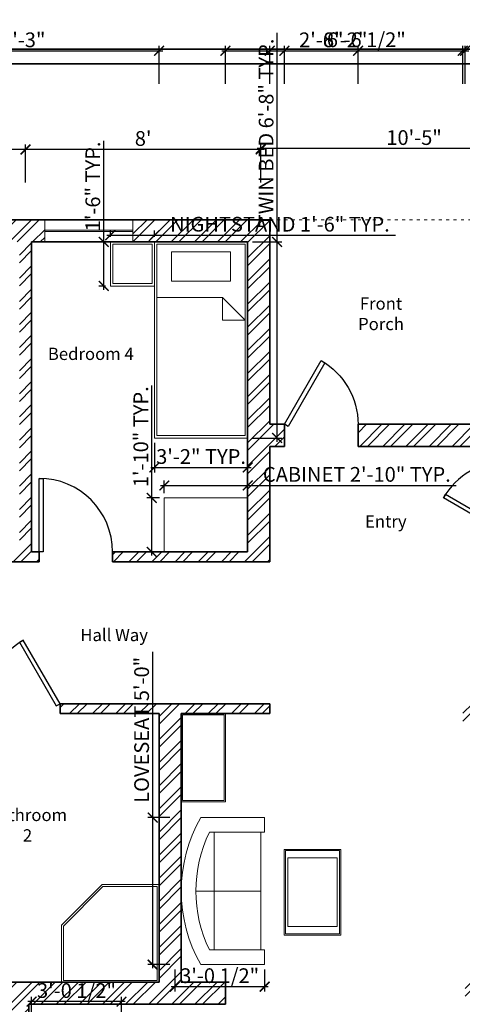
# Model space of a CAD drawing. Units: inches. Extents: x 163 to 947, y 159 to 804.
# Tile 3 of 5: x 444 to 625, y 403 to 804. Entities that reach past the tile are written whole.
import ezdxf

# ---------------------------------------------------------------- set-up
doc = ezdxf.new("R2010")
doc.units = ezdxf.units.IN
doc.linetypes.add('ACAD_ISO03W100', pattern=[30, 12, -18])
for name, color, linetype, lineweight in [('A-ANNO-TTLB', 7, 'Continuous', 35), ('A-AREA-IDEN', 7, 'Continuous', 18), ('A-FLOR-FIXT', 121, 'Continuous', 18), ('A-ROOF-OVHD', 7, 'ACAD_ISO03W100', 18), ('Dimensions', 7, 'Continuous', 18), ('Doors', 160, 'Continuous', 25), ('Furniture', 40, 'Continuous', 18), ('Wall Hatch', 214, 'Continuous', 13), ('Walls', 222, 'Continuous', 35), ('Windows', 132, 'Continuous', 18)]:
    doc.layers.add(name, color=color, linetype=linetype, lineweight=lineweight)
doc.styles.get("Standard").update_dxf_attribs({"font": 'arial.ttf'})
doc.dimstyles.new('ISO-25', dxfattribs={"dimtxt": 6, "dimasz": 4, "dimexe": 2, "dimexo": 2, "dimtad": 1, "dimdec": 1, "dimlunit": 3, "dimtxsty": 'Standard', "dimblk": 'ARCHTICK', "dimcen": 0, "dimdle": 1.5, "dimadec": 0, "dimazin": 0, "dimtfac": 1, "dimtdec": 1, "dimtmove": 0, "dimatfit": 3, "dimfxl": 13.5, "dimfxlon": 1, "dimarcsym": 0})

# ---------------------------------------------------------------- blocks, each defined once
blk = doc.blocks.new('_ArchTick')
at = {"color": 0, "linetype": 'ByBlock', "const_width": 0.15}
blk.add_lwpolyline([(-0.5, -0.5), (0.5, 0.5)], dxfattribs=at)
blk = doc.blocks.new('*D4')
at = {"layer": 'Dimensions', "color": 0, "lineweight": -2, "transparency": 16777216}
for p, q in [((669.3, 751.78), (541.3, 751.78)), ((542.8, 738.28), (542.8, 753.78)), ((667.8, 738.28), (667.8, 753.78))]:
    blk.add_line(p, q, dxfattribs=at)
at = {"layer": 'Dimensions', "color": 0, "lineweight": -2, "transparency": 16777216, "xscale": 4, "yscale": 4, "zscale": 4, "rotation": 180}
blk.add_blockref('_ArchTick', (542.8, 751.78), dxfattribs=at)
at = {"layer": 'Dimensions', "color": 0, "lineweight": -2, "transparency": 16777216, "xscale": 4, "yscale": 4, "zscale": 4}
blk.add_blockref('_ArchTick', (667.8, 751.78), dxfattribs=at)
at = {"layer": 'Dimensions', "color": 0, "transparency": 16777216, "insert": (605.3, 755.47), "char_height": 6, "attachment_point": 5}
blk.add_mtext('10\'-5"', dxfattribs=at)
blk = doc.blocks.new('*D5')
at = {"layer": 'Dimensions', "color": 0, "lineweight": -2, "transparency": 16777216}
for p, q in [((544.3, 751.41), (445.3, 751.41)), ((446.8, 737.91), (446.8, 753.41)), ((542.8, 737.91), (542.8, 753.41))]:
    blk.add_line(p, q, dxfattribs=at)
at = {"layer": 'Dimensions', "color": 0, "lineweight": -2, "transparency": 16777216, "xscale": 4, "yscale": 4, "zscale": 4, "rotation": 180}
blk.add_blockref('_ArchTick', (446.8, 751.41), dxfattribs=at)
at = {"layer": 'Dimensions', "color": 0, "lineweight": -2, "transparency": 16777216, "xscale": 4, "yscale": 4, "zscale": 4}
blk.add_blockref('_ArchTick', (542.8, 751.41), dxfattribs=at)
at = {"layer": 'Dimensions', "color": 0, "transparency": 16777216, "insert": (494.8, 755.1), "char_height": 6, "attachment_point": 5}
blk.add_mtext("8'", dxfattribs=at)
blk = doc.blocks.new('*D6')
at = {"layer": 'Dimensions', "color": 0, "lineweight": -2, "transparency": 16777216}
for p, q in [((448.3, 751.36), (353.3, 751.36)), ((354.8, 737.86), (354.8, 753.36)), ((446.8, 737.86), (446.8, 753.36))]:
    blk.add_line(p, q, dxfattribs=at)
at = {"layer": 'Dimensions', "color": 0, "lineweight": -2, "transparency": 16777216, "xscale": 4, "yscale": 4, "zscale": 4, "rotation": 180}
blk.add_blockref('_ArchTick', (354.8, 751.36), dxfattribs=at)
at = {"layer": 'Dimensions', "color": 0, "lineweight": -2, "transparency": 16777216, "xscale": 4, "yscale": 4, "zscale": 4}
blk.add_blockref('_ArchTick', (446.8, 751.36), dxfattribs=at)
at = {"layer": 'Dimensions', "color": 0, "transparency": 16777216, "insert": (400.8, 755.05), "char_height": 6, "attachment_point": 5}
blk.add_mtext('7\'-8"', dxfattribs=at)
blk = doc.blocks.new('*U20')
for p, q in [((0, 0), (0, -4)), ((30, 0), (30, -4))]:
    blk.add_line(p, q)
blk.add_lwpolyline([(0, 0), (0, 30), (1.75, 30), (1.75, 0)], close=True)
blk.add_arc((0, 0), 30, 0, 90)
blk = doc.blocks.new('*U21')
for p, q in [((0, 0), (0, -4)), ((30, 0), (30, -4))]:
    blk.add_line(p, q)
blk.add_lwpolyline([(0, 0), (15, 25.98), (16.52, 25.11), (1.52, -0.87)], close=True)
blk.add_arc((0, 0), 30, 0, 60)
blk = doc.blocks.new('*U24')
for p, q in [((0, 0), (0, -4)), ((-30, 0), (-30, -4))]:
    blk.add_line(p, q)
blk.add_lwpolyline([(0, 0), (-15, 25.98), (-16.52, 25.11), (-1.52, -0.88)], close=True)
blk.add_arc((0, 0), 30, 120, 180)
blk = doc.blocks.new('*U25')
for p, q in [((-30, 0), (-30, 4)), ((0, 0), (0, 4))]:
    blk.add_line(p, q)
blk.add_lwpolyline([(0, 0), (-15, -25.98), (-16.52, -25.11), (-1.52, 0.87)], close=True)
blk.add_arc((0, 0), 30, 180, 240)
blk = doc.blocks.new('Sofa - Roundback Loveseat 5 ft.')
for p, q in [((0, -32.44198), (0, -5.99998)), ((-24, -33.99998), (-24, -11.46958)), ((24.00004, -33.99998), (24.00004, -11.46958)), ((-23.9998, -13.38178), (23.99986, -13.38178)), ((-24, -32.44198), (24.00004, -32.44198))]:
    blk.add_line(p, q)
for points in [[(-24, -33.99998), (-30, -33.99998), (-30, -7.99998)], [(30.00004, -7.99998), (30.00004, -33.99998), (24.00004, -33.99998)]]:
    blk.add_lwpolyline(points)
for centre, radius, start, end in [((0, -60.24998), 60.24998, 60.13715, 119.8628), ((0, -61.38438), 55.38444, 64.32083, 115.6792)]:
    blk.add_arc(centre, radius, start, end)
blk = doc.blocks.new('WIN-36IN')
for p, q in [((0, 9.03), (0, 0)), ((35.98, 9.03), (35.98, 0)), ((0, 4.76), (35.98, 4.76)), ((0, 4.26), (35.98, 4.26))]:
    blk.add_line(p, q)
blk = doc.blocks.new('BED-TWIN')
for p, q in [((1, 57.33), (27.7, 57.33)), ((27.7, 57.33), (37, 48.04)), ((27.7, 48.04), (27.7, 57.33)), ((37, 48.04), (27.7, 48.04))]:
    blk.add_line(p, q)
for points in [[(0, 0), (38, 0), (38, 80), (0, 80)], [(1, 1), (37, 1), (37, 79), (1, 79)], [(7, 64), (31, 64), (31, 76), (7, 76)]]:
    blk.add_lwpolyline(points, close=True)
blk = doc.blocks.new('NIGHTSTAND-18IN')
for points in [[(0, 0), (18, 0), (18, 18), (0, 18)], [(1, 1), (17, 1), (17, 17), (1, 17)]]:
    blk.add_lwpolyline(points, close=True)
blk = doc.blocks.new('BEDROOM-CABINET-34X22')
blk.add_lwpolyline([(0, 0), (34, 0), (34, 22), (0, 22)], close=True)
blk = doc.blocks.new('*D72')
at = {"layer": 'Dimensions', "color": 0, "lineweight": -2, "transparency": 16777216}
for p, q in [((549.42, 713.71), (549.42, 798.99)), ((539.42, 713.71), (551.42, 713.71)), ((549.42, 632.21), (549.42, 713.71)), ((539.42, 633.71), (551.42, 633.71))]:
    blk.add_line(p, q, dxfattribs=at)
at = {"layer": 'Dimensions', "color": 0, "lineweight": -2, "transparency": 16777216, "xscale": 4, "yscale": 4, "zscale": 4}
for p, rotation in [((549.42, 713.71), 90), ((549.42, 633.71), 270)]:
    blk.add_blockref('_ArchTick', p, dxfattribs=dict(at, rotation=rotation))
at = {"layer": 'Dimensions', "color": 0, "transparency": 16777216, "insert": (545.73, 758.35), "char_height": 6, "attachment_point": 5, "rotation": 90}
blk.add_mtext('TWIN BED 6\'-8" TYP.', dxfattribs=at)
blk = doc.blocks.new('*D73')
at = {"layer": 'Dimensions', "color": 0, "lineweight": -2, "transparency": 16777216}
for p, q in [((499.42, 631.71), (499.42, 619.71)), ((537.42, 631.71), (537.42, 619.71)), ((497.92, 621.71), (538.92, 621.71))]:
    blk.add_line(p, q, dxfattribs=at)
at = {"layer": 'Dimensions', "color": 0, "lineweight": -2, "transparency": 16777216, "xscale": 4, "yscale": 4, "zscale": 4, "rotation": 180}
blk.add_blockref('_ArchTick', (499.42, 621.71), dxfattribs=at)
at = {"layer": 'Dimensions', "color": 0, "lineweight": -2, "transparency": 16777216, "xscale": 4, "yscale": 4, "zscale": 4}
blk.add_blockref('_ArchTick', (537.42, 621.71), dxfattribs=at)
at = {"layer": 'Dimensions', "color": 0, "transparency": 16777216, "insert": (518.42, 625.4), "char_height": 6, "attachment_point": 5}
blk.add_mtext('3\'-2" TYP.', dxfattribs=at)
blk = doc.blocks.new('*D74')
at = {"layer": 'Dimensions', "color": 0, "lineweight": -2, "transparency": 16777216}
for p, q in [((479.92, 716.41), (499.42, 716.41)), ((481.42, 715.71), (481.42, 718.41)), ((499.42, 715.71), (499.42, 718.41)), ((499.42, 716.41), (597.76, 716.41))]:
    blk.add_line(p, q, dxfattribs=at)
at = {"layer": 'Dimensions', "color": 0, "lineweight": -2, "transparency": 16777216, "xscale": 4, "yscale": 4, "zscale": 4, "rotation": 180}
blk.add_blockref('_ArchTick', (481.42, 716.41), dxfattribs=at)
at = {"layer": 'Dimensions', "color": 0, "lineweight": -2, "transparency": 16777216, "xscale": 4, "yscale": 4, "zscale": 4}
blk.add_blockref('_ArchTick', (499.42, 716.41), dxfattribs=at)
at = {"layer": 'Dimensions', "color": 0, "transparency": 16777216, "insert": (550.59, 720.13), "char_height": 6, "attachment_point": 5}
blk.add_mtext('NIGHTSTAND 1\'-6" TYP.', dxfattribs=at)
blk = doc.blocks.new('*D75')
at = {"layer": 'Dimensions', "color": 0, "lineweight": -2, "transparency": 16777216}
for p, q in [((478.72, 713.71), (478.72, 754.96)), ((479.42, 713.71), (476.72, 713.71)), ((478.72, 694.21), (478.72, 713.71)), ((479.42, 695.71), (476.72, 695.71))]:
    blk.add_line(p, q, dxfattribs=at)
at = {"layer": 'Dimensions', "color": 0, "lineweight": -2, "transparency": 16777216, "xscale": 4, "yscale": 4, "zscale": 4}
for p, rotation in [((478.72, 713.71), 90), ((478.72, 695.71), 270)]:
    blk.add_blockref('_ArchTick', p, dxfattribs=dict(at, rotation=rotation))
at = {"layer": 'Dimensions', "color": 0, "transparency": 16777216, "insert": (475.03, 736.33), "char_height": 6, "attachment_point": 5, "rotation": 90}
blk.add_mtext('1\'-6" TYP.', dxfattribs=at)
blk = doc.blocks.new('*D76')
at = {"layer": 'Dimensions', "color": 0, "lineweight": -2, "transparency": 16777216}
for p, q in [((501.92, 614.38), (537.42, 614.38)), ((503.42, 611.28), (503.42, 616.38)), ((537.42, 611.28), (537.42, 616.38)), ((537.42, 614.38), (622.49, 614.38))]:
    blk.add_line(p, q, dxfattribs=at)
at = {"layer": 'Dimensions', "color": 0, "lineweight": -2, "transparency": 16777216, "xscale": 4, "yscale": 4, "zscale": 4, "rotation": 180}
blk.add_blockref('_ArchTick', (503.42, 614.38), dxfattribs=at)
at = {"layer": 'Dimensions', "color": 0, "lineweight": -2, "transparency": 16777216, "xscale": 4, "yscale": 4, "zscale": 4}
blk.add_blockref('_ArchTick', (537.42, 614.38), dxfattribs=at)
at = {"layer": 'Dimensions', "color": 0, "transparency": 16777216, "insert": (581.95, 618.11), "char_height": 6, "attachment_point": 5}
blk.add_mtext('CABINET 2\'-10" TYP.', dxfattribs=at)
blk = doc.blocks.new('*D77')
at = {"layer": 'Dimensions', "color": 0, "lineweight": -2, "transparency": 16777216}
for p, q in [((498.32, 609.28), (498.32, 655.2)), ((501.42, 609.28), (496.32, 609.28)), ((498.32, 585.78), (498.32, 609.28)), ((501.42, 587.28), (496.32, 587.28))]:
    blk.add_line(p, q, dxfattribs=at)
at = {"layer": 'Dimensions', "color": 0, "lineweight": -2, "transparency": 16777216, "xscale": 4, "yscale": 4, "zscale": 4}
for p, rotation in [((498.32, 609.28), 90), ((498.32, 587.28), 270)]:
    blk.add_blockref('_ArchTick', p, dxfattribs=dict(at, rotation=rotation))
at = {"layer": 'Dimensions', "color": 0, "transparency": 16777216, "insert": (494.63, 634.24), "char_height": 6, "attachment_point": 5, "rotation": 90}
blk.add_mtext('1\'-10" TYP.', dxfattribs=at)
blk = doc.blocks.new('*D79')
at = {"layer": 'Dimensions', "color": 0, "lineweight": -2, "transparency": 16777216}
for p, q in [((449.28, 393.27), (449.28, 405.87)), ((485.95, 393.27), (485.95, 405.87)), ((487.45, 403.87), (447.78, 403.87))]:
    blk.add_line(p, q, dxfattribs=at)
at = {"layer": 'Dimensions', "color": 0, "lineweight": -2, "transparency": 16777216, "xscale": 4, "yscale": 4, "zscale": 4, "rotation": 180}
blk.add_blockref('_ArchTick', (449.28, 403.87), dxfattribs=at)
at = {"layer": 'Dimensions', "color": 0, "lineweight": -2, "transparency": 16777216, "xscale": 4, "yscale": 4, "zscale": 4}
blk.add_blockref('_ArchTick', (485.95, 403.87), dxfattribs=at)
at = {"layer": 'Dimensions', "color": 0, "transparency": 16777216, "insert": (467.61, 407.6), "char_height": 6, "attachment_point": 5}
blk.add_mtext('3\'-0 1/2"', dxfattribs=at)
blk = doc.blocks.new('*D80')
at = {"layer": 'Dimensions', "color": 0, "lineweight": -2, "transparency": 16777216}
for p, q in [((498.68, 478.94), (498.68, 546.46)), ((505.68, 478.94), (496.68, 478.94)), ((498.68, 417.44), (498.68, 478.94)), ((505.68, 418.94), (496.68, 418.94))]:
    blk.add_line(p, q, dxfattribs=at)
at = {"layer": 'Dimensions', "color": 0, "lineweight": -2, "transparency": 16777216, "xscale": 4, "yscale": 4, "zscale": 4}
for p, rotation in [((498.68, 478.94), 90), ((498.68, 418.94), 270)]:
    blk.add_blockref('_ArchTick', p, dxfattribs=dict(at, rotation=rotation))
at = {"layer": 'Dimensions', "color": 0, "transparency": 16777216, "insert": (494.95, 514.7), "char_height": 6, "attachment_point": 5, "rotation": 90}
blk.add_mtext('LOVESEAT 5\'-0"', dxfattribs=at)
blk = doc.blocks.new('*D81')
at = {"layer": 'Dimensions', "color": 0, "lineweight": -2, "transparency": 16777216}
for p, q in [((507.68, 416.94), (507.68, 407.94)), ((544.34, 416.94), (544.34, 407.94)), ((545.84, 409.94), (506.18, 409.94))]:
    blk.add_line(p, q, dxfattribs=at)
at = {"layer": 'Dimensions', "color": 0, "lineweight": -2, "transparency": 16777216, "xscale": 4, "yscale": 4, "zscale": 4, "rotation": 180}
blk.add_blockref('_ArchTick', (507.68, 409.94), dxfattribs=at)
at = {"layer": 'Dimensions', "color": 0, "lineweight": -2, "transparency": 16777216, "xscale": 4, "yscale": 4, "zscale": 4}
blk.add_blockref('_ArchTick', (544.34, 409.94), dxfattribs=at)
at = {"layer": 'Dimensions', "color": 0, "transparency": 16777216, "insert": (526.01, 413.67), "char_height": 6, "attachment_point": 5}
blk.add_mtext('3\'-0 1/2"', dxfattribs=at)
blk = doc.blocks.new('*D91')
at = {"layer": 'Dimensions', "color": 0, "lineweight": -2, "transparency": 16777216}
for p, q in [((389, 791.65), (502.82, 791.65)), ((390.5, 778.15), (390.5, 793.65)), ((501.32, 778.15), (501.32, 793.65))]:
    blk.add_line(p, q, dxfattribs=at)
at = {"layer": 'Dimensions', "color": 0, "lineweight": -2, "transparency": 16777216, "xscale": 4, "yscale": 4, "zscale": 4, "rotation": 180}
blk.add_blockref('_ArchTick', (390.5, 791.65), dxfattribs=at)
at = {"layer": 'Dimensions', "color": 0, "lineweight": -2, "transparency": 16777216, "xscale": 4, "yscale": 4, "zscale": 4}
blk.add_blockref('_ArchTick', (501.32, 791.65), dxfattribs=at)
at = {"layer": 'Dimensions', "color": 0, "transparency": 16777216, "insert": (445.91, 795.34), "char_height": 6, "attachment_point": 5}
blk.add_mtext('9\'-3"', dxfattribs=at)
blk = doc.blocks.new('*D92')
at = {"layer": 'Dimensions', "color": 0, "lineweight": -2, "transparency": 16777216}
for p, q in [((175.19, 410.29), (175.19, 522.85)), ((188.69, 521.35), (173.19, 521.35)), ((188.69, 411.79), (173.19, 411.79))]:
    blk.add_line(p, q, dxfattribs=at)
at = {"layer": 'Dimensions', "color": 0, "lineweight": -2, "transparency": 16777216, "xscale": 4, "yscale": 4, "zscale": 4}
for p, rotation in [((175.19, 521.35), 90), ((175.19, 411.79), 270)]:
    blk.add_blockref('_ArchTick', p, dxfattribs=dict(at, rotation=rotation))
at = {"layer": 'Dimensions', "color": 0, "transparency": 16777216, "insert": (171.47, 466.57), "char_height": 6, "attachment_point": 5, "rotation": 90}
blk.add_mtext('9\'-1 1/2"', dxfattribs=at)
blk = doc.blocks.new('*D95')
at = {"layer": 'Dimensions', "color": 0, "lineweight": -2, "transparency": 16777216}
for p, q in [((550.94, 791.65), (583.93, 791.65)), ((552.44, 778.15), (552.44, 793.65)), ((582.43, 778.15), (582.43, 793.65))]:
    blk.add_line(p, q, dxfattribs=at)
at = {"layer": 'Dimensions', "color": 0, "lineweight": -2, "transparency": 16777216, "xscale": 4, "yscale": 4, "zscale": 4, "rotation": 180}
blk.add_blockref('_ArchTick', (552.44, 791.65), dxfattribs=at)
at = {"layer": 'Dimensions', "color": 0, "lineweight": -2, "transparency": 16777216, "xscale": 4, "yscale": 4, "zscale": 4}
blk.add_blockref('_ArchTick', (582.43, 791.65), dxfattribs=at)
at = {"layer": 'Dimensions', "color": 0, "transparency": 16777216, "insert": (567.43, 795.34), "char_height": 6, "attachment_point": 5}
blk.add_mtext('2\'-6"', dxfattribs=at)
blk = doc.blocks.new('*D99')
at = {"layer": 'Dimensions', "color": 0, "lineweight": -2, "transparency": 16777216}
for p, q in [((526.83, 791.65), (627.6, 791.65)), ((528.33, 778.15), (528.33, 793.65)), ((626.1, 778.15), (626.1, 793.65))]:
    blk.add_line(p, q, dxfattribs=at)
at = {"layer": 'Dimensions', "color": 0, "lineweight": -2, "transparency": 16777216, "xscale": 4, "yscale": 4, "zscale": 4, "rotation": 180}
blk.add_blockref('_ArchTick', (528.33, 791.65), dxfattribs=at)
at = {"layer": 'Dimensions', "color": 0, "lineweight": -2, "transparency": 16777216, "xscale": 4, "yscale": 4, "zscale": 4}
blk.add_blockref('_ArchTick', (626.1, 791.65), dxfattribs=at)
at = {"layer": 'Dimensions', "color": 0, "transparency": 16777216, "insert": (577.22, 795.34), "char_height": 6, "attachment_point": 5}
blk.add_mtext('8\'-2"', dxfattribs=at)
blk = doc.blocks.new('*D100')
at = {"layer": 'Dimensions', "color": 0, "lineweight": -2, "transparency": 16777216}
for p, q in [((544.94, 791.65), (626.67, 791.65)), ((546.44, 778.15), (546.44, 793.65)), ((625.17, 778.15), (625.17, 793.65))]:
    blk.add_line(p, q, dxfattribs=at)
at = {"layer": 'Dimensions', "color": 0, "lineweight": -2, "transparency": 16777216, "xscale": 4, "yscale": 4, "zscale": 4, "rotation": 180}
blk.add_blockref('_ArchTick', (546.44, 791.65), dxfattribs=at)
at = {"layer": 'Dimensions', "color": 0, "lineweight": -2, "transparency": 16777216, "xscale": 4, "yscale": 4, "zscale": 4}
blk.add_blockref('_ArchTick', (625.17, 791.65), dxfattribs=at)
at = {"layer": 'Dimensions', "color": 0, "transparency": 16777216, "insert": (585.81, 795.38), "char_height": 6, "attachment_point": 5}
blk.add_mtext('6\'-6 1/2"', dxfattribs=at)

msp = doc.modelspace()

# ---------------------------------------------------------------- hatches: boundary and pattern name
at = {"layer": 'Wall Hatch'}
h = msp.add_hatch(dxfattribs=at)
h.set_pattern_fill('ANSI32', color=256, scale=0.7)
h.paths.add_polyline_path([(271.66, 713.71), (308.91, 713.71), (308.91, 722.73), (262.64, 722.73), (262.64, 565.31), (271.66, 565.31), (271.66, 583.27), (310.31, 583.27), (310.31, 587.28), (271.66, 587.28)])
h.paths.add_polyline_path([(357.32, 713.71), (400.68, 713.71), (400.68, 722.73), (344.89, 722.73), (344.89, 713.71), (352.3, 713.71), (352.3, 587.28), (340.31, 587.28), (340.31, 583.27), (387.9, 583.27), (387.9, 580.28), (391.92, 580.28), (391.92, 583.27), (411.3, 583.27), (411.3, 587.28), (357.32, 587.28)])
h.paths.add_polyline_path([(454.65, 722.73), (436.66, 722.73), (436.66, 713.71), (444.3, 713.71), (444.3, 587.28), (441.3, 587.28), (441.3, 583.27), (452.32, 583.27), (452.32, 587.28), (449.32, 587.28), (449.32, 713.71), (454.65, 713.71)])
h.paths.add_polyline_path([(546.44, 722.73), (490.63, 722.73), (490.63, 713.71), (537.42, 713.71), (537.42, 587.28), (482.32, 587.28), (482.32, 583.27), (546.44, 583.27), (546.44, 630.27), (552.44, 630.27), (552.44, 639.3), (546.44, 639.3)])
h.paths.add_polyline_path([(271.66, 529.33), (262.64, 529.33), (262.64, 402.77), (290.54, 402.77), (290.54, 411.79), (271.66, 411.79)])
h.paths.add_polyline_path([(344.49, 408.77), (344.51, 411.79), (326.52, 411.79), (326.52, 402.77), (344.49, 402.77)])
h.paths.add_polyline_path([(528.33, 411.79), (510.34, 411.79), (510.34, 521.35), (546.44, 521.35), (546.44, 525.36), (460.92, 525.36), (460.9, 525.35), (460.9, 521.35), (501.32, 521.35), (501.32, 411.79), (390.5, 411.79), (390.5, 521.35), (430.9, 521.35), (430.9, 525.36), (390.5, 525.36), (390.5, 541.96), (386.49, 541.96), (386.49, 411.79), (380.49, 411.79), (380.49, 402.77), (439.11, 402.77), (439.11, 392.26), (448.14, 392.26), (448.14, 402.77), (528.33, 402.77)])
h.paths.add_polyline_path([(448.14, 356.28), (439.11, 356.28), (439.11, 338.29), (448.14, 338.29)])
h.paths.add_polyline_path([(542.45, 294.79), (448.14, 294.79), (448.14, 302.31), (439.11, 302.31), (439.11, 285.77), (542.45, 285.77)])
h.paths.add_polyline_path([(596.42, 294.79), (578.43, 294.79), (578.43, 285.77), (596.42, 285.77)])
h.paths.add_polyline_path([(653.12, 402.77), (659.11, 402.77), (659.11, 408.77), (659.11, 411.79), (626.1, 411.79), (626.1, 402.77), (644.09, 402.77), (644.09, 294.79), (632.4, 294.79), (632.4, 285.77), (653.12, 285.77)])
h.paths.add_polyline_path([(738.49, 630.27), (844.6, 630.27), (844.6, 603.27), (853.62, 603.27), (853.62, 722.73), (663.29, 722.73), (663.29, 677.29), (672.32, 677.29), (672.32, 713.71), (777.6, 713.71), (777.6, 669.29), (783.62, 669.29), (783.62, 713.71), (844.6, 713.71), (844.6, 636.29), (783.62, 636.29), (783.62, 639.29), (777.6, 639.29), (777.6, 636.29), (672.32, 636.29), (672.32, 645.29), (663.29, 645.29), (663.29, 639.3), (582.43, 639.3), (582.43, 630.27), (643.22, 630.27), (643.22, 624.27), (648.23, 624.27), (648.23, 630.27), (732.47, 630.27), (732.47, 547.43), (648.23, 547.43), (648.23, 594.27), (643.22, 594.27), (643.22, 525.36), (625.17, 525.36), (625.17, 517.34), (648.23, 517.34), (648.23, 541.41), (729.47, 541.41), (729.47, 517.34), (738.49, 517.34)])
h.paths.add_polyline_path([(853.62, 567.29), (844.6, 567.29), (844.6, 489.33), (853.62, 489.33)])
h.paths.add_polyline_path([(853.62, 453.35), (844.6, 453.35), (844.6, 411.79), (826.3, 411.79), (826.3, 402.77), (853.62, 402.77)])
h.paths.add_polyline_path([(790.32, 411.79), (772.33, 411.79), (772.33, 402.77), (790.32, 402.77)])
h.paths.add_polyline_path([(736.35, 411.79), (695.11, 411.79), (695.11, 402.77), (736.35, 402.77)])

# ---------------------------------------------------------------- linework, layer by layer
at = {"layer": 'A-ANNO-TTLB'}
for points in [[(163.29, 792.35), (947.45, 792.35), (947.45, 158.54), (163.29, 158.54)], [(169.29, 786.35), (941.45, 786.35), (941.45, 164.54), (169.29, 164.54)]]:
    msp.add_lwpolyline(points, close=True, dxfattribs=at)
at = {"layer": 'A-FLOR-FIXT'}
for points in [[(461.53, 435), (461.53, 411.79), (501.32, 411.79), (501.32, 451.58), (478.11, 451.58)], [(462.28, 434.69), (462.28, 412.54), (500.57, 412.54), (500.57, 450.83), (478.42, 450.83)]]:
    msp.add_lwpolyline(points, close=True, dxfattribs=at)
at = {"layer": 'A-ROOF-OVHD', "ltscale": 0.1}
msp.add_line((546.44, 722.73), (663.29, 722.73), dxfattribs=at)
at = {"layer": 'Furniture'}
for p, q in [((553.87, 462.46), (553.87, 434.46)), ((573.87, 462.46), (553.87, 462.46)), ((573.87, 434.46), (573.87, 462.46)), ((553.87, 434.46), (573.87, 434.46))]:
    msp.add_line(p, q, dxfattribs=at)
for points in [[(510.34, 485.35), (528.34, 485.35), (528.34, 521.35), (510.34, 521.35)], [(510.84, 485.85), (527.84, 485.85), (527.84, 520.85), (510.84, 520.85)], [(575.37, 430.96), (575.37, 465.96), (552.37, 465.96), (552.37, 430.96)], [(574.87, 431.46), (574.87, 465.46), (552.87, 465.46), (552.87, 431.46)]]:
    msp.add_lwpolyline(points, close=True, dxfattribs=at)
at = {"layer": 'Walls'}
for p, q in [((546.44, 722.73), (262.64, 722.73)), ((546.44, 639.3), (546.44, 722.73)), ((449.32, 713.71), (449.32, 587.28)), ((537.42, 713.71), (449.32, 713.71)), ((537.42, 587.28), (537.42, 713.71)), ((552.44, 639.3), (546.44, 639.3)), ((552.44, 639.3), (552.44, 630.27)), ((663.29, 639.3), (582.43, 639.3)), ((582.43, 639.3), (582.43, 630.27)), ((546.44, 583.27), (546.44, 630.27)), ((552.44, 630.27), (546.44, 630.27)), ((643.22, 630.27), (582.43, 630.27)), ((452.32, 587.28), (449.32, 587.28)), ((452.32, 587.28), (452.32, 583.27)), ((537.42, 587.28), (482.32, 587.28)), ((482.32, 587.28), (482.32, 583.27)), ((452.32, 583.27), (441.3, 583.27)), ((546.44, 583.27), (482.32, 583.27)), ((546.44, 525.36), (460.9, 525.36)), ((460.9, 525.36), (460.9, 521.35)), ((546.44, 521.35), (546.44, 525.36)), ((501.32, 521.35), (460.9, 521.35)), ((501.32, 411.79), (501.32, 521.35)), ((510.34, 411.79), (510.34, 521.35)), ((546.44, 521.35), (510.34, 521.35)), ((501.32, 411.79), (390.5, 411.79)), ((528.33, 411.79), (510.34, 411.79)), ((528.33, 411.79), (528.33, 402.77)), ((448.14, 402.77), (448.14, 294.79)), ((528.33, 402.77), (448.14, 402.77))]:
    msp.add_line(p, q, dxfattribs=at)

# ---------------------------------------------------------------- block references
at = {"layer": 'Doors', "xscale": -1}
for name, p in [('*U24', (552.43, 639.3)), ('*U21', (460.9, 525.35))]:
    msp.add_blockref(name, p, dxfattribs=at)
at = {"layer": 'Doors', "rotation": 270}
msp.add_blockref('*U25', (643.22, 594.27), dxfattribs=at)
at = {"layer": 'Doors'}
msp.add_blockref('*U20', (452.32, 587.27), dxfattribs=at)
at = {"layer": 'Furniture'}
for name, p in [('NIGHTSTAND-18IN', (481.42, 695.71)), ('BED-TWIN', (499.42, 633.71)), ('BEDROOM-CABINET-34X22', (503.42, 587.28))]:
    msp.add_blockref(name, p, dxfattribs=at)
at = {"layer": 'Furniture', "rotation": 90}
msp.add_blockref('Sofa - Roundback Loveseat 5 ft.', (510.34, 448.94), dxfattribs=at)
at = {"layer": 'Windows'}
msp.add_blockref('WIN-36IN', (454.65, 713.7), dxfattribs=at)

# ---------------------------------------------------------------- texts
at = {"layer": 'A-AREA-IDEN', "char_height": 5, "attachment_point": 1}
for s, insert in [('\\pxqc;{\\fTimes New Roman|b0|i0|c0|p18;Front Porch}', (573.77, 691.05)), ('\\pxqc;{\\fTimes New Roman|b0|i0|c0|p18;Bedroom 4}', (455.4, 670.54)), ('\\pxqc;{\\fTimes New Roman|b0|i0|c0|p18;Entry}', (575.72, 602.21)), ('\\pxqc;{\\fTimes New Roman|b0|i0|c0|p18;Hall Way}', (464.92, 555.88)), ('\\pxqc;{\\fTimes New Roman|b0|i0|c0|p18;Bathroom 2}', (429.6, 482.49))]:
    msp.add_mtext_dynamic_manual_height_columns(s, width=36.0874, gutter_width=12.5, heights=[0], dxfattribs=dict(at, insert=insert))

# ---------------------------------------------------------------- dimensions: what is measured, and where the dimension line sits
at = {"layer": 'Dimensions'}
for base, p1, p2, override, picture, middle in [((625.17, 791.65), (546.44, 525.36), (625.17, 525.36), {"dimdec": 1, "dimlfac": 1, "dimrnd": 0, "dimzin": 1, "dimdsep": 46, "dimlunit": 4, "dimfrac": 2}, '*D100', (585.81, 795.38)), ((501.32, 791.65), (390.5, 521.35), (501.32, 521.35), {"dimdec": 1, "dimlfac": 1, "dimrnd": 0, "dimzin": 1, "dimdsep": 46, "dimlunit": 4, "dimfrac": 2}, '*D91', (445.91, 795.34)), ((626.1, 791.65), (528.33, 411.79), (626.1, 411.79), {"dimdec": 1, "dimlfac": 1, "dimrnd": 0, "dimzin": 1, "dimdsep": 46, "dimlunit": 4, "dimfrac": 2}, '*D99', (577.22, 795.34)), ((582.43, 791.65), (552.44, 639.3), (582.43, 639.3), {"dimdec": 1, "dimlfac": 1, "dimrnd": 0, "dimzin": 1, "dimdsep": 46, "dimlunit": 4, "dimfrac": 2}, '*D95', (567.43, 795.34)), ((354.8, 751.36), (446.8, 724.34), (354.8, 724.34), {"dimclrd": 0, "dimclre": 0, "dimclrt": 0}, '*D6', (400.8, 755.05)), ((446.8, 751.41), (542.8, 724.34), (446.8, 724.34), {"dimclrd": 0, "dimclre": 0, "dimclrt": 0}, '*D5', (494.8, 755.1)), ((542.8, 751.78), (667.8, 724.34), (542.8, 724.34), {"dimclrd": 0, "dimclre": 0, "dimclrt": 0}, '*D4', (605.3, 755.47))]:
    dim = msp.add_linear_dim(base=base, p1=p1, p2=p2, dimstyle='ISO-25', override=override, dxfattribs=at)
    dim.commit()
    dim.dimension.update_dxf_attribs({"geometry": picture, "text_midpoint": middle})
for base, p1, p2, text, picture, middle in [((549.42, 713.71), (537.42, 633.71), (537.42, 713.71), 'TWIN BED <> TYP.', '*D72', (545.73, 758.35)), ((478.72, 713.71), (481.42, 695.71), (481.42, 713.71), '<> TYP.', '*D75', (475.03, 736.33)), ((498.32, 609.28), (503.42, 587.28), (503.42, 609.28), '<> TYP.', '*D77', (494.63, 634.24)), ((498.68, 478.94), (507.68, 418.94), (507.68, 478.94), 'LOVESEAT <>', '*D80', (494.95, 514.7))]:
    dim = msp.add_linear_dim(base=base, p1=p1, p2=p2, angle=90, text=text, dimstyle='ISO-25', override={"dimdec": 1, "dimlfac": 1, "dimrnd": 0, "dimzin": 1, "dimdsep": 46, "dimlunit": 4, "dimfrac": 2}, dxfattribs=at)
    dim.commit()
    dim.dimension.update_dxf_attribs({"geometry": picture, "text_midpoint": middle})
for base, p1, p2, text, picture, middle in [((499.42, 716.41), (481.42, 713.71), (499.42, 713.71), 'NIGHTSTAND <> TYP.', '*D74', (550.59, 720.13)), ((537.42, 621.71), (499.42, 633.71), (537.42, 633.71), '<> TYP.', '*D73', (518.42, 625.4)), ((537.42, 614.38), (503.42, 609.28), (537.42, 609.28), 'CABINET <> TYP.', '*D76', (581.95, 618.11))]:
    dim = msp.add_linear_dim(base=base, p1=p1, p2=p2, text=text, dimstyle='ISO-25', override={"dimdec": 1, "dimlfac": 1, "dimrnd": 0, "dimzin": 1, "dimdsep": 46, "dimlunit": 4, "dimfrac": 2}, dxfattribs=at)
    dim.commit()
    dim.dimension.update_dxf_attribs({"geometry": picture, "text_midpoint": middle})
for base, p1, p2, angle, picture, middle in [((175.19, 521.35), (501.32, 411.79), (501.32, 521.35), 90, '*D92', (171.47, 466.57)), ((507.68, 409.94), (544.34, 418.94), (507.68, 418.94), 180, '*D81', (526.01, 413.67)), ((449.28, 403.87), (485.95, 391.27), (449.28, 391.27), 180, '*D79', (467.61, 407.6))]:
    dim = msp.add_linear_dim(base=base, p1=p1, p2=p2, angle=angle, dimstyle='ISO-25', override={"dimdec": 1, "dimlfac": 1, "dimrnd": 0, "dimzin": 1, "dimdsep": 46, "dimlunit": 4, "dimfrac": 2}, dxfattribs=at)
    dim.commit()
    dim.dimension.update_dxf_attribs({"geometry": picture, "text_midpoint": middle})

doc.saveas('drawing.dxf')
